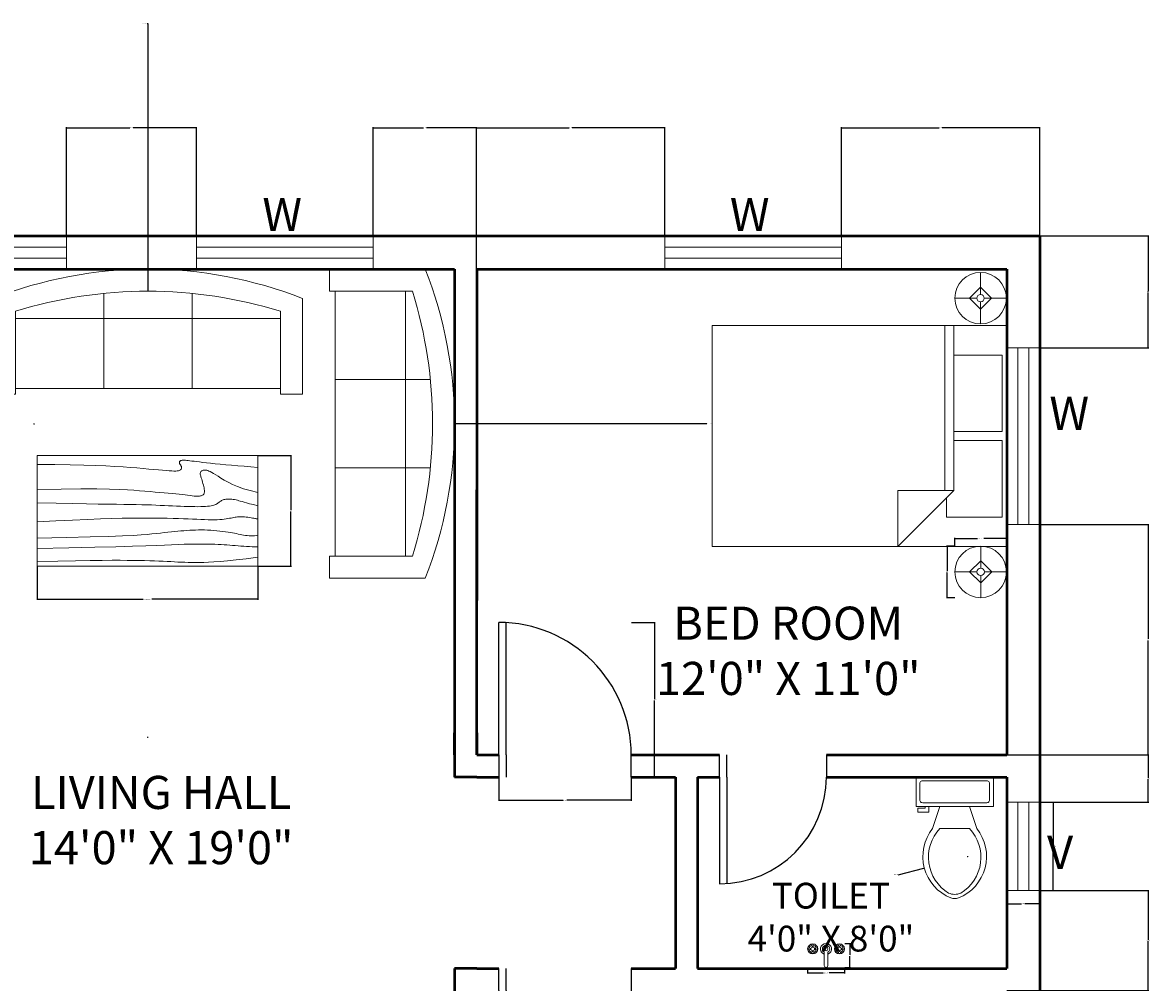
# Model space of a CAD drawing. Units: inches. Extents: x 1727 to 2326, y 1693 to 2164.
# Tile 3 of 3: x 2020 to 2326, y 1904 to 2164. Entities that reach past the tile are written whole.
import ezdxf

# ---------------------------------------------------------------- set-up
doc = ezdxf.new("R2010")
doc.units = ezdxf.units.IN
for name, color, linetype, lineweight in [('A-ANNO-DIMS', 2, 'Continuous', 18), ('A-ANNO-TEXT', 3, 'Continuous', 18), ('A-AREA-IDEN', 7, 'Continuous', 25), ('A-DOOR', 3, 'Continuous', 25), ('A-FLOR-FIXT', 9, 'Continuous', 20), ('A-FURN', 8, 'Continuous', 18), ('A-GLAZ', 4, 'Continuous', 18), ('A-WALL', 7, 'Continuous', 50)]:
    doc.layers.add(name, color=color, linetype=linetype, lineweight=lineweight)
doc.styles.add('Annotative', font='arial.ttf')
doc.styles.get("Standard").update_dxf_attribs({"font": 'arial.ttf'})
doc.dimstyles.get("Standard").update_dxf_attribs({"dimtxt": 0.18, "dimasz": 0.18, "dimexe": 0.18, "dimexo": 0.0625, "dimgap": 0.09, "dimtad": 0, "dimtih": 1, "dimtoh": 1, "dimdec": 4, "dimzin": 0, "dimdsep": 46, "dimtxsty": 'Standard', "dimcen": 0.09, "dimadec": 0, "dimazin": 0, "dimtfac": 1, "dimtdec": 4, "dimtofl": 0, "dimtmove": 0, "dimatfit": 3, "dimfxl": 1, "dimtolj": 1, "dimtzin": 0, "dimarcsym": 0})

# ---------------------------------------------------------------- blocks, each defined once
blk = doc.blocks.new('Bed - Queen')
for p, q in [((0, -80.00003), (0, 0)), ((0, 0), (59.99999, 0)), ((59.99999, 0), (59.99999, -80.00003)), ((7.99999, -1.2), (28.79998, -1.2)), ((7.99999, -14.4), (7.99999, -1.2)), ((28.79998, -1.2), (28.79998, -14.4)), ((31.19999, -1.2), (51.99999, -1.2)), ((31.19999, -14.4), (31.19999, -1.2)), ((51.99999, -1.2), (51.99999, -16.4)), ((0, -14.4), (44.8, -14.4)), ((59.99999, -29.6), (44.8, -14.4)), ((44.8, -14.4), (44.8, -29.6)), ((44.8, -16.8), (0, -16.8)), ((51.99999, -16.4), (46.79936, -16.4)), ((44.8, -29.6), (59.99999, -29.6)), ((59.99999, -80.00003), (0, -80.00003))]:
    blk.add_line(p, q)
blk = doc.blocks.new('Lamp - Table')
for p, q in [((0, 7), (0, 1)), ((-1, 0), (-7, 0)), ((0, 3), (-3, 0)), ((-3, 0), (0, -3)), ((3, 0), (0, 3)), ((0, -3), (3, 0)), ((1, 0), (7, 0)), ((0, -1), (0, -7))]:
    blk.add_line(p, q)
for radius in [7, 1]:
    blk.add_circle((0, 0), radius)
blk = doc.blocks.new('Sofa - Roundback 7 ft.')
for p, q in [((-12.00002, -32.4421), (-12.00003, -6.5971)), ((11.99997, -32.4421), (11.99998, -6.5971)), ((-36.000027, -34), (-36.000027, -11.4696)), ((35.99998, -34), (35.99998, -11.4696)), ((-35.999844, -13.3819), (35.9998, -13.3819)), ((-36.000027, -32.4421), (35.99998, -32.4421))]:
    blk.add_line(p, q)
for points in [[(-36.000027, -34), (-42.000027, -34), (-42.000027, -8)], [(41.99998, -8), (41.99998, -34), (35.99998, -34)]]:
    blk.add_lwpolyline(points)
for centre, radius, start, end in [((0, -114.25), 114.25, 68.43141, 111.5686), ((-0.00001, -127.1968), 121.1968, 72.72033, 107.2797)]:
    blk.add_arc(centre, radius, start, end)
blk = doc.blocks.new('Table - Rectangular Woodgrain 60 x 30 in.')
for p, q in [((0, 0), (0, -30)), ((60, 0), (0, 0)), ((60, -30), (60, 0)), ((0, -30), (60, -30))]:
    blk.add_line(p, q)
for points in [[(0, -2.4), (4.8155, -2.418), (9.0302, -2.4688), (12.709, -2.5477), (15.9167, -2.65), (18.7181, -2.7711), (21.1781, -2.9063), (23.3616, -3.0508), (25.3333, -3.2), (27.1477, -3.3495), (28.8172, -3.4958), (30.3437, -3.636), (31.7291, -3.7667), (32.9756, -3.8849), (34.0849, -3.9875), (35.059, -4.0714), (35.9, -4.1334), (36.6114, -4.1711), (37.2041, -4.1854), (37.6906, -4.1779), (38.0833, -4.15), (38.3948, -4.1034), (38.6375, -4.0396), (38.8239, -3.9602), (38.9666, -3.8667), (39.0764, -3.7608), (39.1573, -3.6448), (39.2116, -3.521), (39.2416, -3.3917), (39.2498, -3.2593), (39.2385, -3.1261), (39.21, -2.9944), (39.1666, -2.8667), (39.111, -2.7447), (39.0468, -2.6281), (38.978, -2.5163), (38.9083, -2.4083), (38.8418, -2.3035), (38.7823, -2.201), (38.7337, -2.1001), (38.7, -2), (38.6844, -1.9003), (38.6875, -1.8021), (38.7094, -1.707), (38.75, -1.6167), (38.8094, -1.5326), (38.8875, -1.4563), (38.9844, -1.3893), (39.1, -1.3333), (39.2351, -1.2896), (39.3937, -1.2583), (39.5804, -1.2396), (39.8, -1.2333), (40.057, -1.2396), (40.3562, -1.2583), (40.7023, -1.2896), (41.1, -1.3333), (41.5547, -1.3895), (42.0755, -1.4573), (42.6721, -1.5361), (43.3542, -1.625), (44.1316, -1.7233), (45.014, -1.8302), (46.0114, -1.9449), (47.1333, -2.0667), (48.3862, -2.1947), (49.7625, -2.3281), (51.2513, -2.4663), (52.8416, -2.6083), (54.5226, -2.7535), (56.2833, -2.9011), (58.1127, -3.0501), (60, -3.2)], [(0, -9.2), (6.5759, -9.0858), (11.9385, -9.0365), (16.2527, -9.0418), (19.6833, -9.0917), (22.3952, -9.1759), (24.5531, -9.2844), (26.322, -9.4069), (27.8666, -9.5333), (29.3241, -9.6553), (30.7203, -9.7719), (32.0532, -9.8837), (33.3208, -9.9917), (34.5213, -10.0965), (35.6526, -10.199), (36.7128, -10.2999), (37.7, -10.4), (38.6129, -10.4996), (39.4531, -10.5969), (40.223, -10.6895), (40.925, -10.775), (41.5613, -10.8512), (42.1344, -10.9156), (42.6465, -10.966), (43.1, -11), (43.4976, -11.0158), (43.8437, -11.0136), (44.143, -10.9942), (44.4, -10.9583), (44.6195, -10.9069), (44.8062, -10.8406), (44.9648, -10.7603), (45.1, -10.6667), (45.2155, -10.5598), (45.3114, -10.4365), (45.3871, -10.2929), (45.4416, -10.125), (45.4743, -9.929), (45.4844, -9.7011), (45.4709, -9.4371), (45.4333, -9.1333), (45.3716, -8.7883), (45.2896, -8.4104), (45.1919, -8.0107), (45.0833, -7.6), (44.9685, -7.1893), (44.8521, -6.7896), (44.7388, -6.4117), (44.6333, -6.0667), (44.54, -5.7628), (44.4614, -5.4979), (44.4001, -5.2675), (44.3583, -5.0667), (44.3384, -4.8909), (44.3427, -4.7354), (44.3736, -4.5956), (44.4333, -4.4667), (44.5236, -4.3453), (44.6427, -4.2333), (44.7884, -4.1339), (44.9583, -4.05), (45.1501, -3.9849), (45.3614, -3.9417), (45.59, -3.9234), (45.8333, -3.9333), (46.0915, -3.9749), (46.3734, -4.0531), (46.6906, -4.1736), (47.0542, -4.3417), (47.4756, -4.5629), (47.9661, -4.8427), (48.5372, -5.1866), (49.2, -5.6), (49.9676, -6.0844), (50.8594, -6.625), (51.8965, -7.2031), (53.1, -7.8), (54.491, -8.3969), (56.0906, -8.975), (57.9199, -9.5156), (60, -10)], [(0, -12.8), (5.1847, -12.9322), (9.6213, -13.0323), (13.3963, -13.1059), (16.5958, -13.1583), (19.3063, -13.1952), (21.614, -13.2219), (23.6054, -13.2439), (25.3666, -13.2667), (26.9728, -13.2947), (28.4531, -13.3281), (29.8256, -13.3663), (31.1083, -13.4083), (32.3191, -13.4535), (33.476, -13.501), (34.597, -13.5501), (35.7, -13.6), (36.7984, -13.6497), (37.8875, -13.6979), (38.9578, -13.743), (40, -13.7833), (41.0047, -13.8174), (41.9625, -13.8438), (42.864, -13.8607), (43.7, -13.8667), (44.4631, -13.8604), (45.1552, -13.8417), (45.7801, -13.8104), (46.3416, -13.7667), (46.8439, -13.7104), (47.2906, -13.6417), (47.6858, -13.5604), (48.0333, -13.4667), (48.3375, -13.3608), (48.6042, -13.2448), (48.8396, -13.121), (49.05, -12.9917), (49.2417, -12.8593), (49.4208, -12.7261), (49.5937, -12.5944), (49.7667, -12.4667), (49.9452, -12.3451), (50.1323, -12.2313), (50.3303, -12.1268), (50.5416, -12.0333), (50.7686, -11.9524), (51.0135, -11.8854), (51.2788, -11.8341), (51.5666, -11.8), (51.8785, -11.7843), (52.2116, -11.7865), (52.562, -11.8059), (52.926, -11.8417), (53.2998, -11.8931), (53.6795, -11.9594), (54.0614, -12.0397), (54.4416, -12.1333), (54.8223, -12.2401), (55.2293, -12.3625), (55.6942, -12.5037), (56.2489, -12.6667), (56.9251, -12.8547), (57.7545, -13.0708), (58.7689, -13.3182), (60, -13.6)], [(0, -18), (5.124, -17.7273), (9.6609, -17.5057), (13.6705, -17.3303), (17.2125, -17.1958), (20.3467, -17.0973), (23.1328, -17.0297), (25.6307, -16.9878), (27.9, -16.9667), (29.9928, -16.9617), (31.9302, -16.9703), (33.7254, -16.9907), (35.3917, -17.0208), (36.9423, -17.0588), (38.3906, -17.1026), (39.7499, -17.1503), (41.0333, -17.2), (42.2519, -17.2496), (43.4073, -17.2969), (44.4986, -17.3395), (45.525, -17.375), (46.4858, -17.4012), (47.3802, -17.4156), (48.2074, -17.416), (48.9667, -17.4), (49.6583, -17.3662), (50.2872, -17.3167), (50.8595, -17.2547), (51.3812, -17.1833), (51.8584, -17.1057), (52.2971, -17.025), (52.7034, -16.9443), (53.0833, -16.8667), (53.443, -16.7951), (53.789, -16.7313), (54.128, -16.6768), (54.4666, -16.6334), (54.8115, -16.6024), (55.1693, -16.5854), (55.5465, -16.5841), (55.95, -16.6), (56.3828, -16.6337), (56.8346, -16.6823), (57.2915, -16.7418), (57.7396, -16.8084), (58.165, -16.878), (58.5539, -16.9469), (58.8924, -17.0111), (59.1666, -17.0667), (59.3679, -17.1107), (59.5078, -17.1438), (59.6032, -17.1675), (59.6708, -17.1833), (59.7275, -17.193), (59.7901, -17.1979), (59.8753, -17.1998), (60, -17.2)], [(0, -22.4), (8.0098, -22.2501), (14.4094, -22.1011), (19.4168, -21.9535), (23.25, -21.8083), (26.1269, -21.6663), (28.2656, -21.5281), (29.884, -21.3947), (31.2, -21.2667), (32.3967, -21.1448), (33.5172, -21.0292), (34.5697, -20.9198), (35.5625, -20.8167), (36.5037, -20.7198), (37.4015, -20.6292), (38.2642, -20.5448), (39.1, -20.4667), (39.9164, -20.3951), (40.7187, -20.3313), (41.5117, -20.2768), (42.3, -20.2333), (43.0883, -20.2024), (43.8812, -20.1854), (44.6836, -20.1841), (45.5, -20.2), (46.3328, -20.234), (47.1747, -20.2844), (48.0163, -20.3488), (48.8479, -20.425), (49.66, -20.5106), (50.4429, -20.6031), (51.1872, -20.7004), (51.8833, -20.8), (52.5246, -20.8999), (53.1166, -20.9995), (53.6681, -21.0983), (54.1875, -21.1958), (54.6834, -21.2919), (55.1646, -21.3859), (55.6394, -21.4777), (56.1167, -21.5667), (56.6028, -21.6515), (57.0961, -21.7266), (57.5929, -21.7852), (58.0896, -21.8208), (58.5823, -21.8268), (59.0674, -21.7964), (59.5412, -21.723), (60, -21.6)], [(0, -25.2), (8.6355, -25.0504), (15.7026, -24.9031), (21.4049, -24.7606), (25.9458, -24.625), (29.529, -24.4988), (32.3578, -24.3844), (34.6359, -24.284), (36.5667, -24.2), (38.3213, -24.1341), (39.9417, -24.0854), (41.437, -24.0523), (42.8167, -24.0333), (44.0901, -24.0268), (45.2667, -24.0313), (46.3557, -24.0451), (47.3667, -24.0667), (48.309, -24.0947), (49.1928, -24.1287), (50.0284, -24.168), (50.826, -24.2125), (51.5959, -24.2617), (52.3483, -24.3151), (53.0935, -24.3725), (53.8417, -24.4334), (54.6009, -24.497), (55.3699, -24.561), (56.1454, -24.6226), (56.9239, -24.6792), (57.7021, -24.7279), (58.4764, -24.7662), (59.2435, -24.7911), (60, -24.8)], [(0, -28.8), (5.6867, -28.6681), (10.45, -28.5698), (14.407, -28.5012), (17.675, -28.4584), (20.3711, -28.4374), (22.6125, -28.4344), (24.5164, -28.4455), (26.2, -28.4667), (27.762, -28.4947), (29.2276, -28.5281), (30.6033, -28.5663), (31.8958, -28.6084), (33.1118, -28.6535), (34.2578, -28.7011), (35.3405, -28.7501), (36.3666, -28.8), (37.3443, -28.8497), (38.288, -28.8974), (39.2137, -28.9412), (40.1375, -28.9792), (41.0753, -29.0093), (42.0432, -29.0297), (43.0572, -29.0384), (44.1333, -29.0333), (45.2936, -29.0114), (46.5843, -28.9641), (48.0579, -28.8816), (49.7666, -28.7542), (51.7629, -28.5721), (54.0989, -28.3255), (56.8272, -28.0048), (60, -27.6)]]:
    blk.add_lwpolyline(points)
blk = doc.blocks.new('Toilet - top')
for p, q in [((9.5, -6), (9.5, -2)), ((-10, -8.5), (-8, -8.5)), ((-10, -9.5), (-10, -8.5)), ((-8, -8.5), (-8, -8)), ((-7, -8), (-7, -9.5)), ((-4, -8), (-6, -14)), ((4, -8), (6, -14)), ((-7, -9.5), (-10, -9.5)), ((4, -14), (-4, -14))]:
    blk.add_line(p, q)
blk.add_lwpolyline([(10.5, -8), (10.5, 0), (-10.5, 0), (-10.5, -8)], close=True)
for points in [[(-9.5, -2), (-9.5, -6)], [(8.5, -1), (-8.5, -1)], [(-8.5, -7), (8.5, -7)]]:
    blk.add_lwpolyline(points)
for centre, radius, start, end in [((-8.62, -1.88), 0.884, 81.8699, 188.1301), ((8.62, -1.88), 0.884, 351.8699, 98.1301), ((-8.62, -6.12), 0.884, 171.8699, 278.1301), ((8.62, -6.12), 0.884, 261.8699, 8.1301), ((3.52, -21.58), 12.17, 141.4691, 247.9714), ((4.2, -21.82), 11.33, 136.3677, 238.9468), ((-3.52, -21.58), 12.17, 292.0284, 38.5307), ((-4.2, -21.82), 11.33, 301.053, 43.6321), ((0, -27.88), 4, 245.7318, 294.2682), ((0, -29), 4, 254.8605, 285.1395)]:
    blk.add_arc(centre, radius, start, end)
blk = doc.blocks.new('Faucet - Bathroom top')
for p, q in [((-4.107, 0.125), (-4.375, 0.125)), ((-3.75, 0.4788), (-3.75, 0.75)), ((-3.5, 0.482), (-3.5, 0.75)), ((-3.1461, 0.125), (-2.875, 0.125)), ((3.143, 0.125), (2.875, 0.125)), ((3.5, 0.4788), (3.5, 0.75)), ((3.75, 0.482), (3.75, 0.75)), ((4.1039, 0.125), (4.375, 0.125)), ((-4.1039, -0.125), (-4.375, -0.125)), ((-3.75, -0.4821), (-3.75, -0.75)), ((-3.5, -0.4789), (-3.5, -0.75)), ((-3.143, -0.125), (-2.875, -0.125)), ((-0.5, -0.8639), (-0.5, -4.5)), ((0.5, -4.5), (0.5, -0.8631)), ((3.1461, -0.125), (2.875, -0.125)), ((3.5, -0.4821), (3.5, -0.75)), ((3.75, -0.4789), (3.75, -0.75)), ((4.107, -0.125), (4.375, -0.125))]:
    blk.add_line(p, q)
for centre, radius in [((-3.625, 0), 1.375), ((-4.625, 0), 0.2795), ((-3.625, 0), 0.5), ((-3.625, 1), 0.2795), ((-2.625, 0), 0.2795), ((0, 0), 0.5), ((3.625, 0), 1.375), ((2.625, 0), 0.2795), ((3.625, 0), 0.5), ((3.625, 1), 0.2795), ((4.625, 0), 0.2795), ((-3.625, -1), 0.2795), ((3.625, -1), 0.2795)]:
    blk.add_circle(centre, radius)
for centre, radius, start, end in [((-3.625, 0), 1, 105.2407, 164.2093), ((-3.625, 0), 1, 16.44125, 74.07887), ((0, 0), 1.5, 289.6514, 250.3603), ((0, 0), 1, 300.3431, 239.7554), ((3.625, 0), 1, 106.12, 164.0884), ((3.625, 0), 1, 16.23422, 73.90469), ((-3.625, 0), 1, 196.2342, 253.9047), ((-3.625, 0), 1, 286.12, 344.0884), ((3.625, 0), 1, 196.4413, 254.0789), ((3.625, 0), 1, 285.2407, 344.2093), ((0, -4.5), 0.5, 180, 0)]:
    blk.add_arc(centre, radius, start, end)
blk = doc.blocks.new('WIN-48IN')
for p, q in [((0, 48), (0, 0)), ((9, 48), (0, 48)), ((3, 48), (3, 0)), ((6, 0), (6, 48)), ((9, 0), (9, 48)), ((0, 0), (9, 0))]:
    blk.add_line(p, q)
blk = doc.blocks.new('VENT-24IN')
for p, q in [((0, 24), (0, 0)), ((9, 24), (0, 24)), ((3, 24), (3, 0)), ((6, 0), (6, 24)), ((9, 0), (9, 24)), ((0, 0), (9, 0))]:
    blk.add_line(p, q)
blk = doc.blocks.new('DOOR-SWING-36IN')
for p, q in [((0, 6), (0, 42)), ((2, 6), (2, 42)), ((0, 6), (0, 0)), ((2, 6), (2, 0)), ((36, 0), (36, 6))]:
    blk.add_line(p, q)
blk.add_arc((0, 6), 36, 0, 90)
blk = doc.blocks.new('DOOR-SWING-29IN')
for p, q in [((0, 29), (0, 35)), ((2, 29), (2, 35)), ((29, 35), (29, 29)), ((0, 29), (0, 0)), ((2, 29), (2, 0))]:
    blk.add_line(p, q)
blk.add_arc((0, 29), 29, 270, 0)
blk = doc.blocks.new('*D15')
at = {"layer": 'A-ANNO-DIMS', "color": 0, "lineweight": -2, "transparency": 16777216}
for p, q in [((2273.29, 2022.17), (2273.29, 2024.39)), ((2273.47, 2024.21), (2279.39, 2024.21)), ((2287.11, 2024.21), (2281.19, 2024.21)), ((2287.29, 2022.17), (2287.29, 2024.39))]:
    blk.add_line(p, q, dxfattribs=at)
at = {"layer": 'A-ANNO-DIMS', "color": 0, "transparency": 16777216}
for points in [[(2273.47, 2024.24), (2273.47, 2024.18), (2273.29, 2024.21)], [(2287.11, 2024.24), (2287.11, 2024.18), (2287.29, 2024.21)]]:
    blk.add_solid(points, dxfattribs=at)
at = {"layer": 'Defpoints', "color": 0, "transparency": 16777216}
for p in [(2287.29, 2024.21), (2273.29, 2022.11), (2287.29, 2022.11)]:
    blk.add_point(p, dxfattribs=at)
at = {"layer": 'A-ANNO-DIMS', "color": 0, "transparency": 16777216, "insert": (2280.29, 2024.21), "char_height": 0.18, "attachment_point": 5}
blk.add_mtext('\\A1;LAMP 14 TYP.', dxfattribs=at)
blk = doc.blocks.new('*D16')
at = {"layer": 'A-ANNO-DIMS', "color": 0, "lineweight": -2, "transparency": 16777216}
for p, q in [((2273.23, 2022.11), (2271.01, 2022.11)), ((2271.19, 2021.93), (2271.19, 2015.29)), ((2271.19, 2008.29), (2271.19, 2014.93)), ((2273.23, 2008.11), (2271.01, 2008.11))]:
    blk.add_line(p, q, dxfattribs=at)
at = {"layer": 'A-ANNO-DIMS', "color": 0, "transparency": 16777216}
for points in [[(2271.16, 2021.93), (2271.22, 2021.93), (2271.19, 2022.11)], [(2271.16, 2008.29), (2271.22, 2008.29), (2271.19, 2008.11)]]:
    blk.add_solid(points, dxfattribs=at)
at = {"layer": 'Defpoints', "color": 0, "transparency": 16777216}
for p in [(2271.19, 2022.11), (2273.29, 2022.11), (2273.29, 2008.11)]:
    blk.add_point(p, dxfattribs=at)
at = {"layer": 'A-ANNO-DIMS', "color": 0, "transparency": 16777216, "insert": (2271.19, 2015.11), "char_height": 0.18, "attachment_point": 5}
blk.add_mtext('\\A1;14 TYP.', dxfattribs=at)
blk = doc.blocks.new('*D25')
at = {"layer": 'A-ANNO-DIMS', "color": 0, "lineweight": -2, "transparency": 16777216}
for p, q in [((2233.29, 1907.62), (2233.29, 1906)), ((2243.29, 1907.62), (2243.29, 1906)), ((2233.47, 1906.18), (2237.48, 1906.18)), ((2243.11, 1906.18), (2239.1, 1906.18))]:
    blk.add_line(p, q, dxfattribs=at)
at = {"layer": 'A-ANNO-DIMS', "color": 0, "transparency": 16777216}
for points in [[(2233.47, 1906.21), (2233.47, 1906.15), (2233.29, 1906.18)], [(2243.11, 1906.21), (2243.11, 1906.15), (2243.29, 1906.18)]]:
    blk.add_solid(points, dxfattribs=at)
at = {"layer": 'Defpoints', "color": 0, "transparency": 16777216}
for p in [(2233.29, 1907.68), (2243.29, 1907.68), (2243.29, 1906.18)]:
    blk.add_point(p, dxfattribs=at)
at = {"layer": 'A-ANNO-DIMS', "color": 0, "transparency": 16777216, "insert": (2238.29, 1906.18), "char_height": 0.18, "attachment_point": 5}
blk.add_mtext('\\A1;TAP 10 TYP.', dxfattribs=at)
blk = doc.blocks.new('*D26')
at = {"layer": 'A-ANNO-DIMS', "color": 0, "lineweight": -2, "transparency": 16777216}
for p, q in [((2243.35, 1914.18), (2244.97, 1914.18)), ((2244.79, 1914), (2244.79, 1911.11)), ((2244.79, 1907.86), (2244.79, 1910.75)), ((2243.35, 1907.68), (2244.97, 1907.68))]:
    blk.add_line(p, q, dxfattribs=at)
at = {"layer": 'A-ANNO-DIMS', "color": 0, "transparency": 16777216}
for points in [[(2244.76, 1914), (2244.82, 1914), (2244.79, 1914.18)], [(2244.76, 1907.86), (2244.82, 1907.86), (2244.79, 1907.68)]]:
    blk.add_solid(points, dxfattribs=at)
at = {"layer": 'Defpoints', "color": 0, "transparency": 16777216}
for p in [(2243.29, 1914.18), (2244.79, 1914.18), (2243.29, 1907.68)]:
    blk.add_point(p, dxfattribs=at)
at = {"layer": 'A-ANNO-DIMS', "color": 0, "transparency": 16777216, "insert": (2244.79, 1910.93), "char_height": 0.18, "attachment_point": 5}
blk.add_mtext('\\A1;7 TYP.', dxfattribs=at)
blk = doc.blocks.new('*D27')
at = {"layer": 'A-ANNO-DIMS', "color": 0, "lineweight": -2, "transparency": 16777216}
for p, q in [((2296.44, 1952.55), (2300.15, 1952.55)), ((2299.97, 1952.37), (2299.97, 1940.73)), ((2299.97, 1928.73), (2299.97, 1940.37)), ((2296.44, 1928.55), (2300.15, 1928.55))]:
    blk.add_line(p, q, dxfattribs=at)
at = {"layer": 'A-ANNO-DIMS', "color": 0, "transparency": 16777216}
for points in [[(2299.94, 1952.37), (2300, 1952.37), (2299.97, 1952.55)], [(2299.94, 1928.73), (2300, 1928.73), (2299.97, 1928.55)]]:
    blk.add_solid(points, dxfattribs=at)
at = {"layer": 'Defpoints', "color": 0, "transparency": 16777216}
for p in [(2296.37, 1952.55), (2299.97, 1952.55), (2296.37, 1928.55)]:
    blk.add_point(p, dxfattribs=at)
at = {"layer": 'A-ANNO-DIMS', "color": 0, "transparency": 16777216, "insert": (2299.97, 1940.55), "char_height": 0.18, "attachment_point": 5}
blk.add_mtext('\\A1;VENT 24 TYP.', dxfattribs=at)
blk = doc.blocks.new('*D28')
at = {"layer": 'A-ANNO-DIMS', "color": 0, "lineweight": -2, "transparency": 16777216}
for p, q in [((2287.37, 1928.49), (2287.37, 1924.77)), ((2296.37, 1928.49), (2296.37, 1924.77)), ((2287.55, 1924.95), (2291.41, 1924.95)), ((2296.19, 1924.95), (2292.33, 1924.95))]:
    blk.add_line(p, q, dxfattribs=at)
at = {"layer": 'A-ANNO-DIMS', "color": 0, "transparency": 16777216}
for points in [[(2287.55, 1924.98), (2287.55, 1924.92), (2287.37, 1924.95)], [(2296.19, 1924.98), (2296.19, 1924.92), (2296.37, 1924.95)]]:
    blk.add_solid(points, dxfattribs=at)
at = {"layer": 'Defpoints', "color": 0, "transparency": 16777216}
for p in [(2287.37, 1928.55), (2296.37, 1928.55), (2296.37, 1924.95)]:
    blk.add_point(p, dxfattribs=at)
at = {"layer": 'A-ANNO-DIMS', "color": 0, "transparency": 16777216, "insert": (2291.87, 1924.95), "char_height": 0.18, "attachment_point": 5}
blk.add_mtext('\\A1;9 TYP.', dxfattribs=at)
blk = doc.blocks.new('*D29')
at = {"layer": 'A-ANNO-DIMS', "color": 0, "lineweight": -2, "transparency": 16777216}
for p, q in [((2185.44, 2001.38), (2191.85, 2001.38)), ((2191.67, 2001.2), (2191.67, 1980.56)), ((2191.67, 1959.56), (2191.67, 1980.2)), ((2185.44, 1959.38), (2191.85, 1959.38))]:
    blk.add_line(p, q, dxfattribs=at)
at = {"layer": 'A-ANNO-DIMS', "color": 0, "transparency": 16777216}
for points in [[(2191.64, 2001.2), (2191.7, 2001.2), (2191.67, 2001.38)], [(2191.64, 1959.56), (2191.7, 1959.56), (2191.67, 1959.38)]]:
    blk.add_solid(points, dxfattribs=at)
at = {"layer": 'Defpoints', "color": 0, "transparency": 16777216}
for p in [(2185.37, 2001.38), (2191.67, 2001.38), (2185.37, 1959.38)]:
    blk.add_point(p, dxfattribs=at)
at = {"layer": 'A-ANNO-DIMS', "color": 0, "transparency": 16777216, "insert": (2191.67, 1980.38), "char_height": 0.18, "attachment_point": 5}
blk.add_mtext('\\A1;DOOR 42 TYP.', dxfattribs=at)
blk = doc.blocks.new('*D30')
at = {"layer": 'A-ANNO-DIMS', "color": 0, "lineweight": -2, "transparency": 16777216}
for p, q in [((2149.37, 1959.32), (2149.37, 1952.9)), ((2185.37, 1959.32), (2185.37, 1952.9)), ((2149.55, 1953.08), (2166.84, 1953.08)), ((2185.19, 1953.08), (2167.9, 1953.08))]:
    blk.add_line(p, q, dxfattribs=at)
at = {"layer": 'A-ANNO-DIMS', "color": 0, "transparency": 16777216}
for points in [[(2149.55, 1953.11), (2149.55, 1953.05), (2149.37, 1953.08)], [(2185.19, 1953.11), (2185.19, 1953.05), (2185.37, 1953.08)]]:
    blk.add_solid(points, dxfattribs=at)
at = {"layer": 'Defpoints', "color": 0, "transparency": 16777216}
for p in [(2149.37, 1959.38), (2185.37, 1959.38), (2185.37, 1953.08)]:
    blk.add_point(p, dxfattribs=at)
at = {"layer": 'A-ANNO-DIMS', "color": 0, "transparency": 16777216, "insert": (2167.37, 1953.08), "char_height": 0.18, "attachment_point": 5}
blk.add_mtext('\\A1;36 TYP.', dxfattribs=at)
blk = doc.blocks.new('*D31')
at = {"layer": 'A-ANNO-DIMS', "color": 0, "lineweight": -2, "transparency": 16777216}
for p, q in [((2023.93, 2016.64), (2023.93, 2007.52)), ((2083.93, 2016.64), (2083.93, 2007.52)), ((2024.11, 2007.7), (2052.74, 2007.7)), ((2083.75, 2007.7), (2055.13, 2007.7))]:
    blk.add_line(p, q, dxfattribs=at)
at = {"layer": 'A-ANNO-DIMS', "color": 0, "transparency": 16777216}
for points in [[(2024.11, 2007.73), (2024.11, 2007.67), (2023.93, 2007.7)], [(2083.75, 2007.73), (2083.75, 2007.67), (2083.93, 2007.7)]]:
    blk.add_solid(points, dxfattribs=at)
at = {"layer": 'Defpoints', "color": 0, "transparency": 16777216}
for p in [(2023.93, 2016.7), (2083.93, 2016.7), (2083.93, 2007.7)]:
    blk.add_point(p, dxfattribs=at)
at = {"layer": 'A-ANNO-DIMS', "color": 0, "transparency": 16777216, "insert": (2053.93, 2007.7), "char_height": 0.18, "attachment_point": 5}
blk.add_mtext('\\A1;COFFEE TABLE 60', dxfattribs=at)
blk = doc.blocks.new('*D32')
at = {"layer": 'A-ANNO-DIMS', "color": 0, "lineweight": -2, "transparency": 16777216}
for p, q in [((2084, 2046.7), (2093.11, 2046.7)), ((2092.93, 2046.52), (2092.93, 2031.88)), ((2092.93, 2016.88), (2092.93, 2031.52)), ((2084, 2016.7), (2093.11, 2016.7))]:
    blk.add_line(p, q, dxfattribs=at)
at = {"layer": 'A-ANNO-DIMS', "color": 0, "transparency": 16777216}
for points in [[(2092.9, 2046.52), (2092.96, 2046.52), (2092.93, 2046.7)], [(2092.9, 2016.88), (2092.96, 2016.88), (2092.93, 2016.7)]]:
    blk.add_solid(points, dxfattribs=at)
at = {"layer": 'Defpoints', "color": 0, "transparency": 16777216}
for p in [(2083.93, 2046.7), (2092.93, 2046.7), (2083.93, 2016.7)]:
    blk.add_point(p, dxfattribs=at)
at = {"layer": 'A-ANNO-DIMS', "color": 0, "transparency": 16777216, "insert": (2092.93, 2031.7), "char_height": 0.18, "attachment_point": 5}
blk.add_mtext('\\A1;30', dxfattribs=at)
blk = doc.blocks.new('*D41')
at = {"layer": 'A-ANNO-DIMS', "color": 0, "lineweight": -2, "transparency": 16777216}
for p, q in [((2031.94, 2106.44), (2031.94, 2135.96)), ((2032.12, 2135.78), (2049.13, 2135.78)), ((2067.06, 2135.78), (2050.05, 2135.78)), ((2067.24, 2106.44), (2067.24, 2135.96))]:
    blk.add_line(p, q, dxfattribs=at)
at = {"layer": 'A-ANNO-DIMS', "color": 0, "transparency": 16777216}
for points in [[(2032.12, 2135.81), (2032.12, 2135.75), (2031.94, 2135.78)], [(2067.06, 2135.81), (2067.06, 2135.75), (2067.24, 2135.78)]]:
    blk.add_solid(points, dxfattribs=at)
at = {"layer": 'Defpoints', "color": 0, "transparency": 16777216}
for p in [(2067.24, 2135.78), (2031.94, 2106.38), (2067.24, 2106.38)]:
    blk.add_point(p, dxfattribs=at)
at = {"layer": 'A-ANNO-DIMS', "color": 0, "transparency": 16777216, "insert": (2049.59, 2135.78), "char_height": 0.18, "attachment_point": 5}
blk.add_mtext('\\A1;35.306', dxfattribs=at)
blk = doc.blocks.new('*D42')
at = {"layer": 'A-ANNO-DIMS', "color": 0, "lineweight": -2, "transparency": 16777216}
for p, q in [((2115.24, 2106.44), (2115.24, 2135.96)), ((2115.42, 2135.78), (2128.91, 2135.78)), ((2143.19, 2135.78), (2129.7, 2135.78)), ((2143.37, 2097.44), (2143.37, 2135.96))]:
    blk.add_line(p, q, dxfattribs=at)
at = {"layer": 'A-ANNO-DIMS', "color": 0, "transparency": 16777216}
for points in [[(2115.42, 2135.81), (2115.42, 2135.75), (2115.24, 2135.78)], [(2143.19, 2135.81), (2143.19, 2135.75), (2143.37, 2135.78)]]:
    blk.add_solid(points, dxfattribs=at)
at = {"layer": 'Defpoints', "color": 0, "transparency": 16777216}
for p in [(2143.37, 2135.78), (2115.24, 2106.38), (2143.37, 2097.38)]:
    blk.add_point(p, dxfattribs=at)
at = {"layer": 'A-ANNO-DIMS', "color": 0, "transparency": 16777216, "insert": (2129.31, 2135.78), "char_height": 0.18, "attachment_point": 5}
blk.add_mtext('\\A1;28.13', dxfattribs=at)
blk = doc.blocks.new('*D43')
at = {"layer": 'A-ANNO-DIMS', "color": 0, "lineweight": -2, "transparency": 16777216}
for p, q in [((2143.37, 2097.44), (2143.37, 2135.96)), ((2143.55, 2135.78), (2168.54, 2135.78)), ((2194.31, 2135.78), (2169.32, 2135.78)), ((2194.49, 2106.44), (2194.49, 2135.96))]:
    blk.add_line(p, q, dxfattribs=at)
at = {"layer": 'A-ANNO-DIMS', "color": 0, "transparency": 16777216}
for points in [[(2143.55, 2135.81), (2143.55, 2135.75), (2143.37, 2135.78)], [(2194.31, 2135.81), (2194.31, 2135.75), (2194.49, 2135.78)]]:
    blk.add_solid(points, dxfattribs=at)
at = {"layer": 'Defpoints', "color": 0, "transparency": 16777216}
for p in [(2194.49, 2135.78), (2194.49, 2106.38), (2143.37, 2097.38)]:
    blk.add_point(p, dxfattribs=at)
at = {"layer": 'A-ANNO-DIMS', "color": 0, "transparency": 16777216, "insert": (2168.93, 2135.78), "char_height": 0.18, "attachment_point": 5}
blk.add_mtext('\\A1;51.12', dxfattribs=at)
blk = doc.blocks.new('*D44')
at = {"layer": 'A-ANNO-DIMS', "color": 0, "lineweight": -2, "transparency": 16777216}
for p, q in [((2242.49, 2106.44), (2242.49, 2135.96)), ((2242.67, 2135.78), (2269.04, 2135.78)), ((2296.19, 2135.78), (2269.83, 2135.78)), ((2296.37, 2106.44), (2296.37, 2135.96))]:
    blk.add_line(p, q, dxfattribs=at)
at = {"layer": 'A-ANNO-DIMS', "color": 0, "transparency": 16777216}
for points in [[(2242.67, 2135.81), (2242.67, 2135.75), (2242.49, 2135.78)], [(2296.19, 2135.81), (2296.19, 2135.75), (2296.37, 2135.78)]]:
    blk.add_solid(points, dxfattribs=at)
at = {"layer": 'Defpoints', "color": 0, "transparency": 16777216}
for p in [(2296.37, 2135.78), (2242.49, 2106.38), (2296.37, 2106.38)]:
    blk.add_point(p, dxfattribs=at)
at = {"layer": 'A-ANNO-DIMS', "color": 0, "transparency": 16777216, "insert": (2269.43, 2135.78), "char_height": 0.18, "attachment_point": 5}
blk.add_mtext('\\A1;53.88', dxfattribs=at)
blk = doc.blocks.new('*D45')
at = {"layer": 'A-ANNO-DIMS', "color": 0, "lineweight": -2, "transparency": 16777216}
for p, q in [((2296.44, 2106.38), (2325.95, 2106.38)), ((2325.77, 2106.2), (2325.77, 2091.39)), ((2325.77, 2076.21), (2325.77, 2091.02)), ((2296.44, 2076.03), (2325.95, 2076.03))]:
    blk.add_line(p, q, dxfattribs=at)
at = {"layer": 'A-ANNO-DIMS', "color": 0, "transparency": 16777216}
for points in [[(2325.74, 2106.2), (2325.8, 2106.2), (2325.77, 2106.38)], [(2325.74, 2076.21), (2325.8, 2076.21), (2325.77, 2076.03)]]:
    blk.add_solid(points, dxfattribs=at)
at = {"layer": 'Defpoints', "color": 0, "transparency": 16777216}
for p in [(2296.37, 2106.38), (2296.37, 2076.03), (2325.77, 2076.03)]:
    blk.add_point(p, dxfattribs=at)
at = {"layer": 'A-ANNO-DIMS', "color": 0, "transparency": 16777216, "insert": (2325.77, 2091.21), "char_height": 0.18, "attachment_point": 5}
blk.add_mtext('\\A1;30.35', dxfattribs=at)
blk = doc.blocks.new('*D46')
at = {"layer": 'A-ANNO-DIMS', "color": 0, "lineweight": -2, "transparency": 16777216}
for p, q in [((2296.44, 2028.03), (2325.95, 2028.03)), ((2325.77, 2027.85), (2325.77, 1996.89)), ((2325.77, 1965.56), (2325.77, 1996.52)), ((2287.44, 1965.38), (2325.95, 1965.38))]:
    blk.add_line(p, q, dxfattribs=at)
at = {"layer": 'A-ANNO-DIMS', "color": 0, "transparency": 16777216}
for points in [[(2325.74, 2027.85), (2325.8, 2027.85), (2325.77, 2028.03)], [(2325.74, 1965.56), (2325.8, 1965.56), (2325.77, 1965.38)]]:
    blk.add_solid(points, dxfattribs=at)
at = {"layer": 'Defpoints', "color": 0, "transparency": 16777216}
for p in [(2296.37, 2028.03), (2287.37, 1965.38), (2325.77, 1965.38)]:
    blk.add_point(p, dxfattribs=at)
at = {"layer": 'A-ANNO-DIMS', "color": 0, "transparency": 16777216, "insert": (2325.77, 1996.71), "char_height": 0.18, "attachment_point": 5}
blk.add_mtext('\\A1;62.65', dxfattribs=at)
blk = doc.blocks.new('*D47')
at = {"layer": 'A-ANNO-DIMS', "color": 0, "lineweight": -2, "transparency": 16777216}
for p, q in [((2287.44, 1965.38), (2325.95, 1965.38)), ((2325.77, 1965.2), (2325.77, 1959.15)), ((2325.77, 1952.73), (2325.77, 1958.78)), ((2296.44, 1952.55), (2325.95, 1952.55))]:
    blk.add_line(p, q, dxfattribs=at)
at = {"layer": 'A-ANNO-DIMS', "color": 0, "transparency": 16777216}
for points in [[(2325.74, 1965.2), (2325.8, 1965.2), (2325.77, 1965.38)], [(2325.74, 1952.73), (2325.8, 1952.73), (2325.77, 1952.55)]]:
    blk.add_solid(points, dxfattribs=at)
at = {"layer": 'Defpoints', "color": 0, "transparency": 16777216}
for p in [(2287.37, 1965.38), (2296.37, 1952.55), (2325.77, 1952.55)]:
    blk.add_point(p, dxfattribs=at)
at = {"layer": 'A-ANNO-DIMS', "color": 0, "transparency": 16777216, "insert": (2325.77, 1958.96), "char_height": 0.18, "attachment_point": 5}
blk.add_mtext('\\A1;12.834', dxfattribs=at)
blk = doc.blocks.new('*D48')
at = {"layer": 'A-ANNO-DIMS', "color": 0, "lineweight": -2, "transparency": 16777216}
for p, q in [((2296.44, 1928.55), (2325.95, 1928.55)), ((2325.77, 1928.37), (2325.77, 1915.15)), ((2325.77, 1901.56), (2325.77, 1914.78)), ((2287.44, 1901.38), (2325.95, 1901.38))]:
    blk.add_line(p, q, dxfattribs=at)
at = {"layer": 'A-ANNO-DIMS', "color": 0, "transparency": 16777216}
for points in [[(2325.74, 1928.37), (2325.8, 1928.37), (2325.77, 1928.55)], [(2325.74, 1901.56), (2325.8, 1901.56), (2325.77, 1901.38)]]:
    blk.add_solid(points, dxfattribs=at)
at = {"layer": 'Defpoints', "color": 0, "transparency": 16777216}
for p in [(2296.37, 1928.55), (2287.37, 1901.38), (2325.77, 1901.38)]:
    blk.add_point(p, dxfattribs=at)
at = {"layer": 'A-ANNO-DIMS', "color": 0, "transparency": 16777216, "insert": (2325.77, 1914.96), "char_height": 0.18, "attachment_point": 5}
blk.add_mtext('\\A1;27.166', dxfattribs=at)
blk = doc.blocks.new('*D67')
at = {"layer": 'A-ANNO-DIMS', "color": 0, "lineweight": -2, "transparency": 16777216}
for p, q in [((2053.86, 2164.1), (2054.04, 2164.1)), ((2054.04, 2164.1), (2054.04, 2091.56)), ((2053.95, 1970.18), (2054.13, 1970.18)), ((2054.04, 1970.09), (2054.04, 1970.27))]:
    blk.add_line(p, q, dxfattribs=at)
at = {"layer": 'A-ANNO-DIMS', "color": 0, "transparency": 16777216}
blk.add_solid([(2054.07, 2091.56), (2054.01, 2091.56), (2054.04, 2091.38)], dxfattribs=at)
at = {"layer": 'Defpoints', "color": 0, "transparency": 16777216}
for p in [(2054.04, 2091.38), (2054.04, 1970.18)]:
    blk.add_point(p, dxfattribs=at)
at = {"layer": 'A-ANNO-DIMS', "color": 0, "transparency": 16777216, "insert": (2053.19, 2164.1), "char_height": 0.18, "attachment_point": 5}
blk.add_mtext('\\A1;3X R121.2', dxfattribs=at)
blk = doc.blocks.new('*D68')
at = {"layer": 'A-ANNO-DIMS', "color": 0, "lineweight": -2, "transparency": 16777216}
for p, q in [((2023.04, 2055.38), (2023.22, 2055.38)), ((2023.13, 2055.29), (2023.13, 2055.47)), ((2205.93, 2055.38), (2137.56, 2055.38))]:
    blk.add_line(p, q, dxfattribs=at)
at = {"layer": 'A-ANNO-DIMS', "color": 0, "transparency": 16777216}
blk.add_solid([(2137.56, 2055.41), (2137.56, 2055.35), (2137.38, 2055.38)], dxfattribs=at)
at = {"layer": 'Defpoints', "color": 0, "transparency": 16777216}
for p in [(2023.13, 2055.38), (2137.38, 2055.38)]:
    blk.add_point(p, dxfattribs=at)
at = {"layer": 'A-ANNO-DIMS', "color": 0, "transparency": 16777216, "insert": (2206.67, 2055.38), "char_height": 0.18, "attachment_point": 5}
blk.add_mtext('\\A1;3X R114.25', dxfattribs=at)
blk = doc.blocks.new('*D69')
at = {"layer": 'A-ANNO-DIMS', "color": 0, "lineweight": -2, "transparency": 16777216}
for p, q in [((2276.67, 1937.8), (2276.85, 1937.8)), ((2276.76, 1937.71), (2276.76, 1937.89)), ((2257.92, 1932.85), (2264.81, 1934.66))]:
    blk.add_line(p, q, dxfattribs=at)
at = {"layer": 'A-ANNO-DIMS', "color": 0, "transparency": 16777216}
blk.add_solid([(2264.8, 1934.69), (2264.82, 1934.63), (2264.99, 1934.71)], dxfattribs=at)
at = {"layer": 'Defpoints', "color": 0, "transparency": 16777216}
for p in [(2276.76, 1937.8), (2264.99, 1934.71)]:
    blk.add_point(p, dxfattribs=at)
at = {"layer": 'A-ANNO-DIMS', "color": 0, "transparency": 16777216, "insert": (2257.25, 1932.85), "char_height": 0.18, "attachment_point": 5}
blk.add_mtext('\\A1;4X R12.17', dxfattribs=at)

msp = doc.modelspace()

# ---------------------------------------------------------------- linework, layer by layer
at = {"layer": 'A-WALL'}
for p, q in [((1756.3729, 2106.3813), (2296.3729, 2106.3813)), ((2296.3729, 2106.3813), (2296.3729, 1746.3813)), ((1969.3729, 2097.3813), (2137.3729, 2097.3813)), ((2137.3729, 2097.3813), (2137.3729, 2007.3813)), ((2143.3729, 2097.3813), (2143.3729, 2007.3813)), ((2143.3729, 2097.3813), (2287.3729, 2097.3813)), ((2287.3729, 2097.3813), (2287.3729, 1965.3813)), ((2143.3729, 2007.3813), (2143.3729, 2037.3813)), ((2137.3729, 2007.3813), (2137.3729, 1971.3813)), ((2143.3729, 1971.3813), (2143.3729, 2007.3813)), ((2137.3729, 1965.3813), (2137.3729, 1971.3813)), ((2137.3729, 1971.3813), (2137.3729, 1959.3813)), ((2143.3729, 1965.3813), (2143.3729, 1971.3813)), ((2143.3729, 1965.3813), (2143.3729, 1971.3813)), ((2143.3729, 1971.3813), (2143.3729, 1965.3813)), ((2143.3729, 1965.3813), (2149.3729, 1965.3813)), ((2143.3729, 1965.3813), (2149.3729, 1965.3813)), ((2185.3729, 1965.3813), (2209.3729, 1965.3813)), ((2238.3729, 1965.3813), (2287.3729, 1965.3813)), ((2143.3729, 1959.3813), (2137.3729, 1959.3813)), ((2143.3729, 1959.3813), (2149.3729, 1959.3813)), ((2143.3729, 1959.3813), (2149.3729, 1959.3813)), ((2185.3729, 1959.3813), (2197.3729, 1959.3813)), ((2197.3729, 1959.3813), (2197.3729, 1907.3813)), ((2203.3729, 1959.3813), (2203.3729, 1907.3813)), ((2203.3729, 1959.3813), (2209.3729, 1959.3813)), ((2203.3729, 1959.3813), (2209.3729, 1959.3813)), ((2238.3729, 1959.3813), (2239.3729, 1959.3813)), ((2239.3729, 1959.3813), (2249.5365, 1959.3813)), ((2245.3729, 1959.3813), (2245.3729, 1959.1283)), ((2245.3729, 1959.3813), (2287.3729, 1959.3813)), ((2287.3729, 1959.3813), (2287.3729, 1907.3813)), ((2143.3729, 1907.3813), (2137.3729, 1907.3813)), ((2137.3729, 1907.3813), (2137.3729, 1869.3813)), ((2143.3729, 1907.3813), (2149.3729, 1907.3813)), ((2185.3729, 1907.3813), (2197.3729, 1907.3813)), ((2203.3729, 1907.3813), (2239.3729, 1907.3813)), ((2239.3729, 1907.3813), (2245.3729, 1907.3813)), ((2245.3729, 1907.3813), (2287.3729, 1907.3813))]:
    msp.add_line(p, q, dxfattribs=at)

# ---------------------------------------------------------------- block references
at = {"layer": 'A-DOOR'}
for name, p in [('DOOR-SWING-36IN', (2149.373, 1959.381)), ('DOOR-SWING-29IN', (2209.373, 1930.381))]:
    msp.add_blockref(name, p, dxfattribs=at)
at = {"layer": 'A-DOOR', "extrusion": (0, 0, -1), "zscale": -1, "rotation": 180}
msp.add_blockref('DOOR-SWING-36IN', (-2149.373, 1907.3817), dxfattribs=at)
at = {"layer": 'A-FLOR-FIXT'}
for name, p in [('Toilet - top', (2273.2358, 1959.3813)), ('Faucet - Bathroom top', (2238.2894, 1912.6795))]:
    msp.add_blockref(name, p, dxfattribs=at)
at = {"layer": 'A-FURN'}
for name, p in [('Sofa - Roundback 7 ft.', (2054.0432, 2097.3813)), ('Lamp - Table', (2280.2703, 2089.4816)), ('Table - Rectangular Woodgrain 60 x 30 in.', (2023.9332, 2046.7004)), ('Lamp - Table', (2280.2926, 2015.1087))]:
    msp.add_blockref(name, p, dxfattribs=at)
at = {"layer": 'A-FURN', "rotation": 270}
for name, p in [('Sofa - Roundback 7 ft.', (2137.3793, 2055.3813)), ('Bed - Queen', (2287.3729, 2082.0287))]:
    msp.add_blockref(name, p, dxfattribs=at)
at = {"layer": 'A-GLAZ'}
for p, rotation in [((1983.936, 2106.3812), 270.0000000000012), ((2067.2423, 2106.3812), 270.0000000000014), ((2194.4901, 2106.3812), 270.0000000000014)]:
    msp.add_blockref('WIN-48IN', p, dxfattribs=dict(at, rotation=rotation))
for name, p in [('WIN-48IN', (2287.373, 2028.032)), ('VENT-24IN', (2287.373, 1928.548))]:
    msp.add_blockref(name, p, dxfattribs=at)

# ---------------------------------------------------------------- texts
at = {"layer": 'A-ANNO-TEXT', "char_height": 9, "width": 33.967268, "attachment_point": 1, "style": 'Annotative'}
for s, insert in [('\\pxqc;W', (2073.5589, 2116.7337)), ('\\pxqc;W', (2200.5582, 2116.7141)), ('\\pxqc;W', (2287.3729, 2062.6987)), ('\\pxqc;V', (2284.8805, 1943.4248))]:
    msp.add_mtext(s, dxfattribs=dict(at, insert=insert))
at = {"layer": 'A-AREA-IDEN', "attachment_point": 1, "style": 'Annotative'}
for s, insert, char_height, width in [('\\pxqc;BED ROOM ^J12\'0" X 11\'0"', (2163.0158, 2005.6769), 9, 130.001559), ('\\pxqc;LIVING HALL\\P14\'0" X 19\'0"', (1992.6536, 1959.6987), 9, 130.001559), ('\\pxqc;TOILET \\P4\'0" X 8\'0"', (2213.3291, 1930.6525), 7, 52.544705)]:
    msp.add_mtext(s, dxfattribs=dict(at, insert=insert, char_height=char_height, width=width))

# ---------------------------------------------------------------- dimensions: what is measured, and where the dimension line sits
at = {"layer": 'A-ANNO-DIMS'}
for center, mpoint, text, override, picture, middle in [((2054.0432, 1970.1845), (2054.043, 2091.3813), '3X <>', {"dimdec": 1, "dimlfac": 1, "dimrnd": 0, "dimzin": 0, "dimdsep": 46, "dimlunit": 2}, '*D67', (2053.1906, 2164.0994)), ((2023.1293, 2055.3813), (2137.3793, 2055.381), '3X <>', {"dimdec": 2, "dimlfac": 1, "dimrnd": 0, "dimzin": 0, "dimdsep": 46, "dimlunit": 2}, '*D68', (2205.9293, 2055.3808)), ((2276.7554, 1937.8008), (2264.9857, 1934.7089), '4X <>', {"dimdec": 2, "dimlfac": 1, "dimrnd": 0, "dimzin": 0, "dimdsep": 46, "dimlunit": 2}, '*D69', (2257.9239, 1932.8538))]:
    dim = msp.add_radius_dim(center=center, mpoint=mpoint, text=text, dimstyle='Standard', override=override, dxfattribs=at)
    dim.commit()
    dim.dimension.update_dxf_attribs({"geometry": picture, "text_midpoint": middle, "dimtype": 164})
for base, p1, p2, override, picture, middle in [((2067.2421, 2135.7813), (2031.9357, 2106.3813), (2067.2421, 2106.3813), {"dimdec": 3, "dimlfac": 1, "dimrnd": 0, "dimzin": 0, "dimdsep": 46, "dimlunit": 2}, '*D41', (2049.5889, 2135.7813)), ((2143.3729, 2135.7813), (2115.2421, 2106.3813), (2143.3729, 2097.3813), {"dimdec": 2, "dimlfac": 1, "dimrnd": 0, "dimzin": 0, "dimdsep": 46, "dimlunit": 2}, '*D42', (2129.3075, 2135.7813)), ((2194.4898, 2135.7813), (2143.3729, 2097.3813), (2194.4898, 2106.3813), {"dimdec": 2, "dimlfac": 1, "dimrnd": 0, "dimzin": 0, "dimdsep": 46, "dimlunit": 2}, '*D43', (2168.9314, 2135.7813)), ((2296.3729, 2135.7813), (2242.4898, 2106.3813), (2296.3729, 2106.3813), {"dimdec": 2, "dimlfac": 1, "dimrnd": 0, "dimzin": 0, "dimdsep": 46, "dimlunit": 2}, '*D44', (2269.4314, 2135.7813))]:
    dim = msp.add_linear_dim(base=base, p1=p1, p2=p2, dimstyle='Standard', override=override, dxfattribs=at)
    dim.commit()
    dim.dimension.update_dxf_attribs({"geometry": picture, "text_midpoint": middle})
for base, p1, p2, override, picture, middle in [((2325.7729, 2076.0317), (2296.3729, 2106.3813), (2296.3729, 2076.0317), {"dimdec": 2, "dimlfac": 1, "dimrnd": 0, "dimzin": 0, "dimdsep": 46, "dimlunit": 2}, '*D45', (2325.7729, 2091.2065)), ((2092.9332, 2046.7004), (2083.9332, 2016.7004), (2083.9332, 2046.7004), {"dimdec": 0, "dimlfac": 1, "dimrnd": 0, "dimzin": 0, "dimdsep": 46, "dimlunit": 2}, '*D32', (2092.9332, 2031.7004)), ((2325.7729, 1965.3813), (2296.3729, 2028.0317), (2287.3729, 1965.3813), {"dimdec": 2, "dimlfac": 1, "dimrnd": 0, "dimzin": 0, "dimdsep": 46, "dimlunit": 2}, '*D46', (2325.7729, 1996.7065)), ((2325.7729, 1952.5475), (2287.3729, 1965.3813), (2296.3729, 1952.5475), {"dimdec": 3, "dimlfac": 1, "dimrnd": 0, "dimzin": 0, "dimdsep": 46, "dimlunit": 2}, '*D47', (2325.7729, 1958.9644)), ((2325.7729, 1901.3813), (2296.3729, 1928.5475), (2287.3729, 1901.3813), {"dimdec": 3, "dimlfac": 1, "dimrnd": 0, "dimzin": 0, "dimdsep": 46, "dimlunit": 2}, '*D48', (2325.7729, 1914.9644))]:
    dim = msp.add_linear_dim(base=base, p1=p1, p2=p2, angle=90, dimstyle='Standard', override=override, dxfattribs=at)
    dim.commit()
    dim.dimension.update_dxf_attribs({"geometry": picture, "text_midpoint": middle})
for base, p1, p2, text, picture, middle in [((2287.2926, 2024.2087), (2273.2926, 2022.1087), (2287.2926, 2022.1087), 'LAMP <> TYP.', '*D15', (2280.2926, 2024.2087)), ((2083.9332, 2007.7004), (2023.9332, 2016.7004), (2083.9332, 2016.7004), 'COFFEE TABLE <>', '*D31', (2053.9332, 2007.7004)), ((2185.3729, 1953.0813), (2149.3729, 1959.3813), (2185.3729, 1959.3813), '<> TYP.', '*D30', (2167.3729, 1953.0813)), ((2296.3729, 1924.9475), (2287.3729, 1928.5475), (2296.3729, 1928.5475), '<> TYP.', '*D28', (2291.8729, 1924.9475)), ((2243.2894, 1906.1795), (2233.2894, 1907.6795), (2243.2894, 1907.6795), 'TAP <> TYP.', '*D25', (2238.2894, 1906.1795))]:
    dim = msp.add_linear_dim(base=base, p1=p1, p2=p2, text=text, dimstyle='Standard', override={"dimdec": 0, "dimlfac": 1, "dimrnd": 0, "dimzin": 0, "dimdsep": 46, "dimlunit": 2}, dxfattribs=at)
    dim.commit()
    dim.dimension.update_dxf_attribs({"geometry": picture, "text_midpoint": middle})
for base, p1, p2, text, picture, middle in [((2271.1926, 2022.1087), (2273.2926, 2008.1087), (2273.2926, 2022.1087), '<> TYP.', '*D16', (2271.1926, 2015.1087)), ((2191.6729, 2001.3813), (2185.3729, 1959.3813), (2185.3729, 2001.3813), 'DOOR <> TYP.', '*D29', (2191.6729, 1980.3813)), ((2299.9729, 1952.5475), (2296.3729, 1928.5475), (2296.3729, 1952.5475), 'VENT <> TYP.', '*D27', (2299.9729, 1940.5475)), ((2244.7894, 1914.1796), (2243.2894, 1907.6795), (2243.2894, 1914.1796), '<> TYP.', '*D26', (2244.7894, 1910.9295))]:
    dim = msp.add_linear_dim(base=base, p1=p1, p2=p2, angle=90, text=text, dimstyle='Standard', override={"dimdec": 0, "dimlfac": 1, "dimrnd": 0, "dimzin": 0, "dimdsep": 46, "dimlunit": 2}, dxfattribs=at)
    dim.commit()
    dim.dimension.update_dxf_attribs({"geometry": picture, "text_midpoint": middle})

doc.saveas('drawing.dxf')
